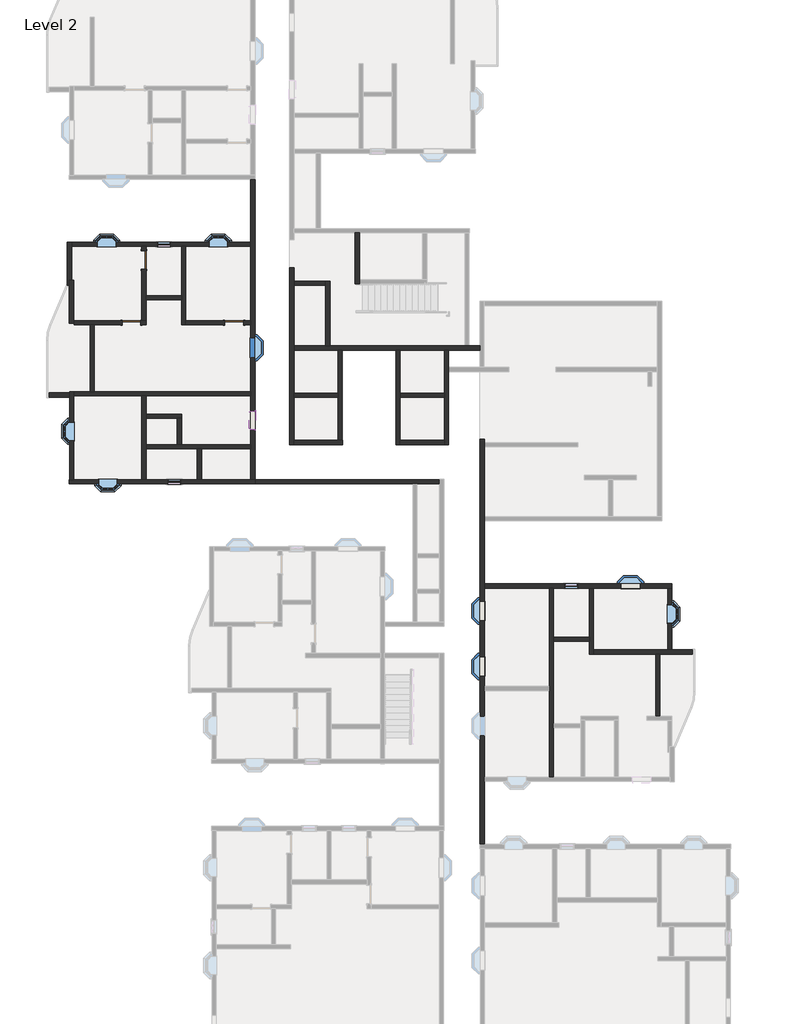
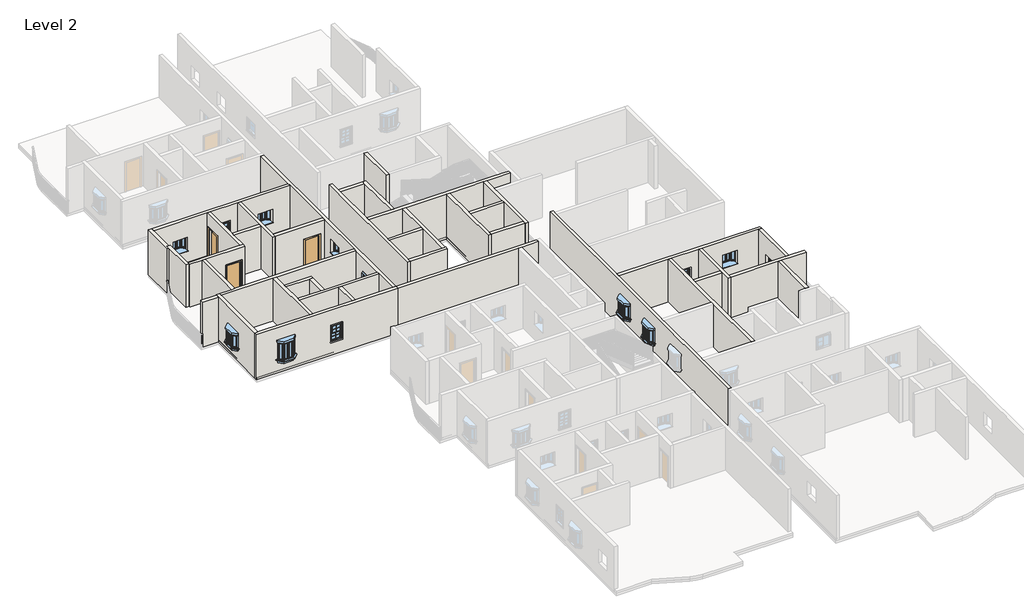
# One storey, part 3 of 14: 40 walls, 13 windows, 3 doors.
# Revit data of these elements (continued)
# Element 26 (IfcWall, "9\"")
#   Top Offset = 0' - 0"
#   Base Offset = 0' - 0"
#   wall height = 10' - 0"
#   Phase Created = New Construction
#   Base Constraint = Level 2
#   Top Constraint = Level 3
#   Materials on its faces: "Default Wall", "Earth"
# Element 27 (IfcWall, "9\"")
#   Top Offset = 0' - 0"
#   Base Offset = 0' - 0"
#   wall height = 10' - 0"
#   Phase Created = New Construction
#   Base Constraint = Level 2
#   Top Constraint = Level 3
#   Materials on its faces: "Default Wall", "Default Mass Interior Wall"
# Element 28 (IfcWall, "9\"")
#   Top Offset = 0' - 0"
#   Base Offset = 0' - 0"
#   wall height = 10' - 0"
#   Phase Created = New Construction
#   Base Constraint = Level 2
#   Top Constraint = Level 3
#   Materials on its faces: "Default Wall"
# Element 29 (IfcWall, "9\"")
#   Top Offset = 0' - 0"
#   Base Offset = 0' - 0"
#   wall height = 10' - 0"
#   Phase Created = New Construction
#   Base Constraint = Level 2
#   Top Constraint = Level 3
#   Materials on its faces: "Default Wall", "Default Mass Interior Wall", "Earth"
# Elements 30, 33, 34, 35, 36, 37, 38, 39, 40, 41 (IfcWall, "9\" w")
#   Top Offset = 0' - 0"
#   Base Offset = 0' - 0"
#   wall height = 10' - 0"
#   Phase Created = New Construction
#   Base Constraint = Level 2
#   Top Constraint = Level 3
#   Materials on its faces: "Default Wall"
# Element 31 (IfcWall, "9\" w")
#   Top Offset = 0' - 0"
#   Base Offset = 0' - 0"
#   wall height = 10' - 0"
#   Phase Created = New Construction
#   Base Constraint = Level 2
#   Top Constraint = Level 3
#   Materials on its faces: "Default Wall", "Earth"
# Element 32 (IfcWall, "9\" w")
#   Top Offset = 0' - 0"
#   Base Offset = 0' - 0"
#   wall height = 10' - 0"
#   Phase Created = New Construction
#   Base Constraint = Level 2
#   Top Constraint = Level 3
#   Materials on its faces: "Default Wall", "Brick, Soldier Course"
# Element 42 (IfcWall, "9\" w")
#   Top Offset = 0' - 0"
#   Base Offset = 0' - 0"
#   wall height = 10' - 0"
#   Phase Created = New Construction
#   Base Constraint = Level 2
#   Top Constraint = Level 3
#   Materials on its faces: "Default Wall", "Wood - Stained"
# Element 43 (IfcWall, "9\" w")
#   Top Offset = 0' - 0"
#   Base Offset = 0' - 0"
#   wall height = 10' - 0"
#   Phase Created = New Construction
#   Base Constraint = Level 2
#   Top Constraint = Level 3
#   Materials on its faces: "Default Wall", "Acoustic Ceiling Tile 24 x 24"
# Element 44 (IfcWindow, "910x1210mm")
#   Mark = "303"
#   Phase Created = New Construction
#   Materials on its faces: "Window Frame", "Glass"
# Element 45 (IfcWindow, "910x910mm")
#   Mark = "91"
#   Phase Created = New Construction
#   Materials on its faces: "Window Frame", "Glass"
# Element 46 (IfcWindow, "910x910mm")
#   Mark = "92"
#   Phase Created = New Construction
#   Materials on its faces: "Window Frame", "Glass"
# Element 47 (IfcWindow, "910x910mm")
#   Mark = "64"
#   Phase Created = New Construction
#   Materials on its faces: "Window Frame", "Glass"
# Element 48 (IfcWindow, "910x910mm")
#   Mark = "65"
#   Phase Created = New Construction
#   Materials on its faces: "Window Frame", "Glass"
# Element 49 (IfcWindow, "910x910mm")
#   Mark = "66"
#   Phase Created = New Construction
#   Materials on its faces: "Window Frame", "Glass"
# Element 50 (IfcWindow, "910x910mm")
#   Mark = "67"
#   Phase Created = New Construction
#   Materials on its faces: "Window Frame", "Glass"
# Element 51 (IfcWindow, "910x910mm")
#   Mark = "89"
#   Phase Created = New Construction
#   Materials on its faces: "Window Frame", "Glass"
# Element 52 (IfcWindow, "910x910mm")
#   Mark = "90"
#   Phase Created = New Construction
#   Materials on its faces: "Window Frame", "Glass"
# Element 53 (IfcWindow, "Window-Double-Hung : 26\" x 42\"")
#   Mark = "113"
#   Window Inset = 0' - 0"
#   Interior Wall Closure = 0' - 1 1/2"
#   Frame Extension = 0' - 1 1/4"
#   Exterior Wall Closure = 0' - 0 1/2"
#   Interior Trim Visibility = yes
#   Indicator Visibility = yes
#   Exterior Trim Visibility = yes
#   Phase Created = New Construction
#   Materials on its faces: "Wood - Stained", "Glass", "Clad - White"
# Element 54 (IfcWindow, "Window-Double-Hung : 26\" x 42\"")
#   Mark = "102"
#   Window Inset = 0' - 0"
#   Interior Wall Closure = 0' - 1 1/2"
#   Frame Extension = 0' - 1 1/4"
#   Exterior Wall Closure = 0' - 0 1/2"
#   Interior Trim Visibility = yes
#   Indicator Visibility = yes
#   Exterior Trim Visibility = yes
#   Phase Created = New Construction
#   Materials on its faces: "Wood - Stained", "Glass", "Clad - White"
# Element 55 (IfcWindow, "Window-Double-Hung : 26\" x 42\"")
#   Mark = "103"
#   Window Inset = 0' - 0"
#   Interior Wall Closure = 0' - 1 1/2"
#   Frame Extension = 0' - 1 1/4"
#   Exterior Wall Closure = 0' - 0 1/2"
#   Interior Trim Visibility = yes
#   Indicator Visibility = yes
#   Exterior Trim Visibility = yes
#   Phase Created = New Construction
#   Materials on its faces: "Wood - Stained", "Glass", "Clad - White"
# Element 56 (IfcWindow, "Windows_Sgl_w-Glazing_Bars : 910x910mm")
#   Mark = "98"
#   Phase Created = New Construction
#   Materials on its faces: "Window Frame", "Glass"
# Materials
#   "Door - Panel": class "Wood", colour RGB 210 159 95, transparency 0, Cost = 0
#   "Door - Frame": colour RGB 118 70 51, transparency 0, Cost = 0
#   "Window Frame": colour RGB 249 249 249, transparency 0
#   "Glass": class "Glass", colour RGB 0 128 192, transparency 0.75, Description = "Soda Lime Glass", Cost = 0
#   "Wood - Stained": class "Wood", colour RGB 224 178 126, transparency 0, Cost = 0
#   "Clad - White": class "Wood", colour RGB 242 242 238, transparency 0, Cost = 0
#   "Default Wall": colour RGB 128 128 128, transparency 0, Cost = 0
#   "Cherry": class "Wood", colour RGB 226 177 128, transparency 0, Description = "Prunus Serotina", Cost = 0
#   "Parking Stripe": class "Paint", colour RGB 250 250 91, transparency 0, Cost = 0
#   "Earth": class "Generic", colour RGB 97 75 62, transparency 0, Description = "Soil", Cost = 0
#   "Default Mass Interior Wall": class "Generic", colour RGB 195 229 126, transparency 0, Cost = 0
#   "Brick, Soldier Course": class "Masonry", colour RGB 170 98 104, transparency 0, Description = "Common brick soldier coursed", Cost = 0
#   "Acoustic Ceiling Tile 24 x 24": class "Generic", colour RGB 232 232 232, transparency 0, Description = "Acoustic Ceiling Tile 24 x 24", Cost = 0
